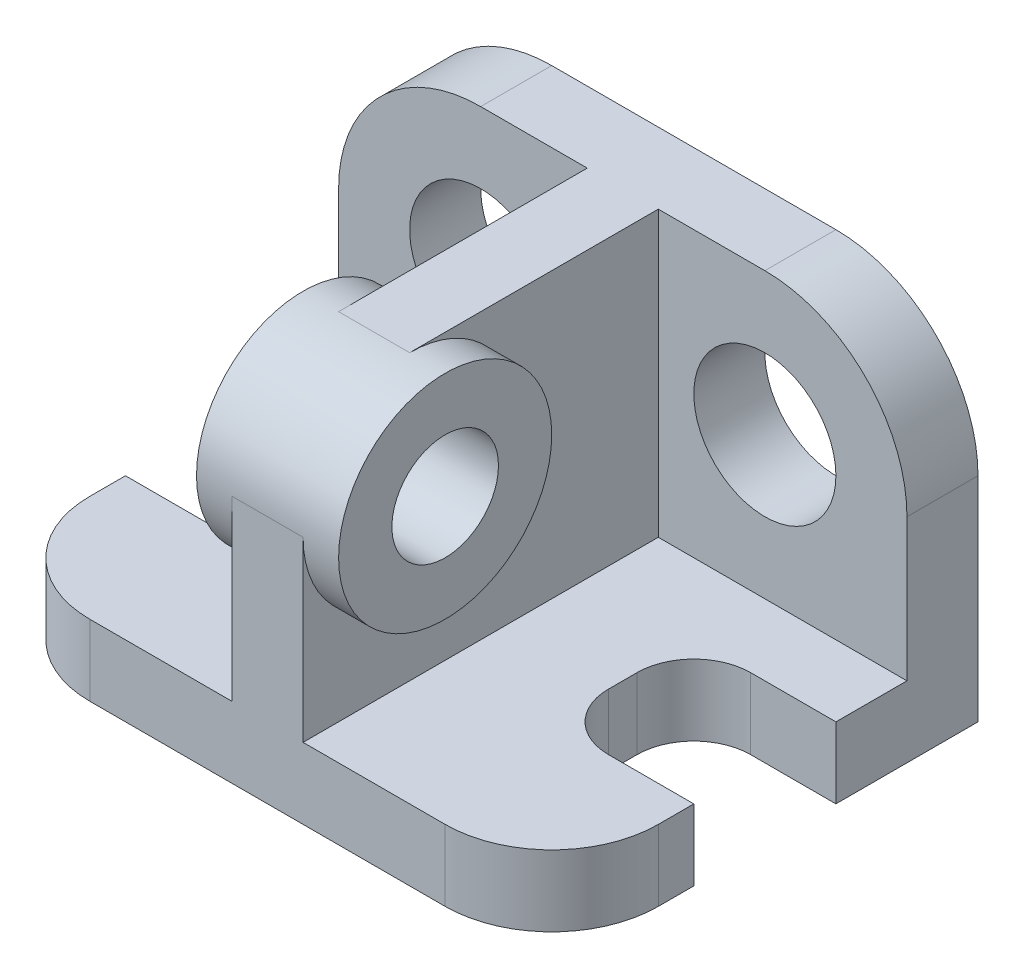
ISO-10303-21;
HEADER;
FILE_DESCRIPTION(('STEP AP214'),'2;1');
FILE_NAME('part.step','',(''),(''),'','','');
FILE_SCHEMA(('AUTOMOTIVE_DESIGN { 1 0 10303 214 1 1 1 1 }'));
ENDSEC;
DATA;
#1=APPLICATION_CONTEXT('core data for automotive mechanical design processes');
#2=APPLICATION_PROTOCOL_DEFINITION('international standard','automotive_design',2000,#1);
#3=PRODUCT_CONTEXT('',#1,'mechanical');
#4=PRODUCT('Part','Part','',(#3));
#5=PRODUCT_RELATED_PRODUCT_CATEGORY('part','',(#4));
#6=PRODUCT_DEFINITION_FORMATION('','',#4);
#7=PRODUCT_DEFINITION_CONTEXT('part definition',#1,'design');
#8=PRODUCT_DEFINITION('design','',#6,#7);
#9=PRODUCT_DEFINITION_SHAPE('','',#8);
#10=(LENGTH_UNIT() NAMED_UNIT(*) SI_UNIT(.MILLI.,.METRE.));
#11=(NAMED_UNIT(*) PLANE_ANGLE_UNIT() SI_UNIT($,.RADIAN.));
#12=(NAMED_UNIT(*) SI_UNIT($,.STERADIAN.) SOLID_ANGLE_UNIT());
#13=UNCERTAINTY_MEASURE_WITH_UNIT(LENGTH_MEASURE(1.E-05),#10,'distance_accuracy_value','');
#14=(GEOMETRIC_REPRESENTATION_CONTEXT(3) GLOBAL_UNCERTAINTY_ASSIGNED_CONTEXT((#13)) GLOBAL_UNIT_ASSIGNED_CONTEXT((#10,
#11,#12)) REPRESENTATION_CONTEXT('',''));
#15=CARTESIAN_POINT('',(0.,0.,0.));
#16=DIRECTION('',(0.,0.,1.));
#17=DIRECTION('',(1.,0.,0.));
#18=AXIS2_PLACEMENT_3D('',#15,#16,#17);
#19=CARTESIAN_POINT('',(-4.,-1.5,6.));
#20=DIRECTION('',(0.,-1.,0.));
#21=DIRECTION('',(0.,0.,-1.));
#22=AXIS2_PLACEMENT_3D('',#19,#20,#21);
#23=PLANE('',#22);
#24=DIRECTION('',(-1.,0.,0.));
#25=VECTOR('',#24,1.);
#26=CARTESIAN_POINT('',(-4.,-1.5,6.));
#27=LINE('',#26,#25);
#28=CARTESIAN_POINT('',(2.5,-1.5,6.));
#29=VERTEX_POINT('',#28);
#30=CARTESIAN_POINT('',(0.5,-1.5,6.));
#31=VERTEX_POINT('',#30);
#32=EDGE_CURVE('E285',#29,#31,#27,.T.);
#33=ORIENTED_EDGE('',*,*,#32,.F.);
#34=CARTESIAN_POINT('',(2.5,-1.5,4.5));
#35=DIRECTION('',(0.,-1.,0.));
#36=DIRECTION('',(0.,0.,-1.));
#37=AXIS2_PLACEMENT_3D('',#34,#35,#36);
#38=CIRCLE('',#37,1.5);
#39=CARTESIAN_POINT('',(4.,-1.5,4.5));
#40=VERTEX_POINT('',#39);
#41=EDGE_CURVE('E260',#29,#40,#38,.F.);
#42=ORIENTED_EDGE('',*,*,#41,.T.);
#43=DIRECTION('',(0.,0.,-1.));
#44=VECTOR('',#43,1.);
#45=CARTESIAN_POINT('',(4.,-1.5,6.));
#46=LINE('',#45,#44);
#47=CARTESIAN_POINT('',(4.,-1.5,4.));
#48=VERTEX_POINT('',#47);
#49=EDGE_CURVE('E283',#40,#48,#46,.T.);
#50=ORIENTED_EDGE('',*,*,#49,.T.);
#51=DIRECTION('',(1.,0.,0.));
#52=VECTOR('',#51,1.);
#53=CARTESIAN_POINT('',(4.,-1.5,4.));
#54=LINE('',#53,#52);
#55=CARTESIAN_POINT('',(2.8,-1.5,4.));
#56=VERTEX_POINT('',#55);
#57=EDGE_CURVE('E443',#56,#48,#54,.T.);
#58=ORIENTED_EDGE('',*,*,#57,.F.);
#59=CARTESIAN_POINT('',(2.8,-1.5,3.2));
#60=DIRECTION('',(0.,1.,0.));
#61=DIRECTION('',(0.,0.,-1.));
#62=AXIS2_PLACEMENT_3D('',#59,#60,#61);
#63=CIRCLE('',#62,0.8);
#64=CARTESIAN_POINT('',(2.,-1.5,3.2));
#65=VERTEX_POINT('',#64);
#66=EDGE_CURVE('E447',#65,#56,#63,.T.);
#67=ORIENTED_EDGE('',*,*,#66,.F.);
#68=DIRECTION('',(0.,0.,1.));
#69=VECTOR('',#68,1.);
#70=CARTESIAN_POINT('',(2.,-1.5,2.8));
#71=LINE('',#70,#69);
#72=CARTESIAN_POINT('',(2.,-1.5,2.8));
#73=VERTEX_POINT('',#72);
#74=EDGE_CURVE('E448',#73,#65,#71,.T.);
#75=ORIENTED_EDGE('',*,*,#74,.F.);
#76=CARTESIAN_POINT('',(2.8,-1.5,2.8));
#77=DIRECTION('',(0.,1.,0.));
#78=DIRECTION('',(0.,0.,-1.));
#79=AXIS2_PLACEMENT_3D('',#76,#77,#78);
#80=CIRCLE('',#79,0.8);
#81=CARTESIAN_POINT('',(2.8,-1.5,2.));
#82=VERTEX_POINT('',#81);
#83=EDGE_CURVE('E454',#82,#73,#80,.T.);
#84=ORIENTED_EDGE('',*,*,#83,.F.);
#85=DIRECTION('',(-1.,0.,0.));
#86=VECTOR('',#85,1.);
#87=CARTESIAN_POINT('',(4.,-1.5,2.));
#88=LINE('',#87,#86);
#89=CARTESIAN_POINT('',(4.,-1.5,2.));
#90=VERTEX_POINT('',#89);
#91=EDGE_CURVE('E406',#90,#82,#88,.T.);
#92=ORIENTED_EDGE('',*,*,#91,.F.);
#93=CARTESIAN_POINT('',(4.,-1.5,1.));
#94=VERTEX_POINT('',#93);
#95=EDGE_CURVE('E293',#90,#94,#46,.T.);
#96=ORIENTED_EDGE('',*,*,#95,.T.);
#97=DIRECTION('',(-1.,0.,0.));
#98=VECTOR('',#97,1.);
#99=CARTESIAN_POINT('',(-4.,-1.5,1.));
#100=LINE('',#99,#98);
#101=CARTESIAN_POINT('',(0.5,-1.5,1.));
#102=VERTEX_POINT('',#101);
#103=EDGE_CURVE('E273',#94,#102,#100,.T.);
#104=ORIENTED_EDGE('',*,*,#103,.T.);
#105=DIRECTION('',(0.,0.,-1.));
#106=VECTOR('',#105,1.);
#107=CARTESIAN_POINT('',(0.5,-1.5,1.));
#108=LINE('',#107,#106);
#109=EDGE_CURVE('E238',#31,#102,#108,.T.);
#110=ORIENTED_EDGE('',*,*,#109,.F.);
#111=EDGE_LOOP('',(#33,#42,#50,#58,#67,#75,#84,#92,#96,#104,#110));
#112=FACE_BOUND('',#111,.T.);
#113=ADVANCED_FACE('F39',(#112),#23,.F.);
#114=CARTESIAN_POINT('',(-2.,0.500000000000001,1.));
#115=DIRECTION('',(0.,0.,-1.));
#116=DIRECTION('',(-1.,0.,0.));
#117=AXIS2_PLACEMENT_3D('',#114,#115,#116);
#118=PLANE('',#117);
#119=CARTESIAN_POINT('',(2.,0.5,1.));
#120=DIRECTION('',(0.,0.,1.));
#121=DIRECTION('',(1.,0.,0.));
#122=AXIS2_PLACEMENT_3D('',#119,#120,#121);
#123=CIRCLE('',#122,1.);
#124=CARTESIAN_POINT('',(3.,0.5,1.));
#125=VERTEX_POINT('',#124);
#126=EDGE_CURVE('E295',#125,#125,#123,.T.);
#127=ORIENTED_EDGE('',*,*,#126,.F.);
#128=EDGE_LOOP('',(#127));
#129=FACE_BOUND('',#128,.T.);
#130=DIRECTION('',(0.,1.,0.));
#131=VECTOR('',#130,1.);
#132=CARTESIAN_POINT('',(0.5,2.5,1.));
#133=LINE('',#132,#131);
#134=CARTESIAN_POINT('',(0.5,2.5,1.));
#135=VERTEX_POINT('',#134);
#136=EDGE_CURVE('E383',#102,#135,#133,.T.);
#137=ORIENTED_EDGE('',*,*,#136,.F.);
#138=ORIENTED_EDGE('',*,*,#103,.F.);
#139=DIRECTION('',(0.,1.,0.));
#140=VECTOR('',#139,1.);
#141=CARTESIAN_POINT('',(4.,0.5,1.));
#142=LINE('',#141,#140);
#143=CARTESIAN_POINT('',(4.,0.5,1.));
#144=VERTEX_POINT('',#143);
#145=EDGE_CURVE('E307',#94,#144,#142,.T.);
#146=ORIENTED_EDGE('',*,*,#145,.T.);
#147=CARTESIAN_POINT('',(2.,0.5,1.));
#148=DIRECTION('',(0.,0.,1.));
#149=DIRECTION('',(1.,0.,0.));
#150=AXIS2_PLACEMENT_3D('',#147,#148,#149);
#151=CIRCLE('',#150,2.);
#152=CARTESIAN_POINT('',(2.,2.5,1.));
#153=VERTEX_POINT('',#152);
#154=EDGE_CURVE('E311',#144,#153,#151,.T.);
#155=ORIENTED_EDGE('',*,*,#154,.T.);
#156=DIRECTION('',(-1.,0.,0.));
#157=VECTOR('',#156,1.);
#158=CARTESIAN_POINT('',(-2.,2.5,1.));
#159=LINE('',#158,#157);
#160=EDGE_CURVE('E314',#153,#135,#159,.T.);
#161=ORIENTED_EDGE('',*,*,#160,.T.);
#162=EDGE_LOOP('',(#137,#138,#146,#155,#161));
#163=FACE_BOUND('',#162,.T.);
#164=ADVANCED_FACE('F481',(#129,#163),#118,.F.);
#165=CARTESIAN_POINT('',(4.,0.5,1.));
#166=DIRECTION('',(-1.,0.,0.));
#167=DIRECTION('',(0.,-1.,0.));
#168=AXIS2_PLACEMENT_3D('',#165,#166,#167);
#169=PLANE('',#168);
#170=DIRECTION('',(0.,1.,0.));
#171=VECTOR('',#170,1.);
#172=CARTESIAN_POINT('',(4.,-2.5,2.));
#173=LINE('',#172,#171);
#174=CARTESIAN_POINT('',(4.,-2.5,2.));
#175=VERTEX_POINT('',#174);
#176=EDGE_CURVE('E431',#175,#90,#173,.T.);
#177=ORIENTED_EDGE('',*,*,#176,.F.);
#178=DIRECTION('',(0.,0.,-1.));
#179=VECTOR('',#178,1.);
#180=CARTESIAN_POINT('',(4.,-2.5,1.));
#181=LINE('',#180,#179);
#182=CARTESIAN_POINT('',(4.,-2.5,0.));
#183=VERTEX_POINT('',#182);
#184=EDGE_CURVE('E325',#175,#183,#181,.T.);
#185=ORIENTED_EDGE('',*,*,#184,.T.);
#186=DIRECTION('',(0.,1.,0.));
#187=VECTOR('',#186,1.);
#188=CARTESIAN_POINT('',(4.,0.5,0.));
#189=LINE('',#188,#187);
#190=CARTESIAN_POINT('',(4.,0.5,0.));
#191=VERTEX_POINT('',#190);
#192=EDGE_CURVE('E306',#183,#191,#189,.T.);
#193=ORIENTED_EDGE('',*,*,#192,.T.);
#194=DIRECTION('',(0.,0.,-1.));
#195=VECTOR('',#194,1.);
#196=CARTESIAN_POINT('',(4.,0.5,1.));
#197=LINE('',#196,#195);
#198=EDGE_CURVE('E244',#144,#191,#197,.T.);
#199=ORIENTED_EDGE('',*,*,#198,.F.);
#200=ORIENTED_EDGE('',*,*,#145,.F.);
#201=ORIENTED_EDGE('',*,*,#95,.F.);
#202=EDGE_LOOP('',(#177,#185,#193,#199,#200,#201));
#203=FACE_BOUND('',#202,.T.);
#204=ADVANCED_FACE('F489',(#203),#169,.F.);
#205=CARTESIAN_POINT('',(-4.,0.500000000000001,1.));
#206=DIRECTION('',(1.,0.,0.));
#207=DIRECTION('',(0.,1.,0.));
#208=AXIS2_PLACEMENT_3D('',#205,#206,#207);
#209=PLANE('',#208);
#210=DIRECTION('',(0.,0.,-1.));
#211=VECTOR('',#210,1.);
#212=CARTESIAN_POINT('',(-4.,-2.5,1.));
#213=LINE('',#212,#211);
#214=CARTESIAN_POINT('',(-4.,-2.5,4.5));
#215=VERTEX_POINT('',#214);
#216=CARTESIAN_POINT('',(-4.,-2.5,4.));
#217=VERTEX_POINT('',#216);
#218=EDGE_CURVE('E336',#215,#217,#213,.T.);
#219=ORIENTED_EDGE('',*,*,#218,.F.);
#220=DIRECTION('',(0.,-1.,0.));
#221=VECTOR('',#220,1.);
#222=CARTESIAN_POINT('',(-4.,0.500000000000001,4.5));
#223=LINE('',#222,#221);
#224=CARTESIAN_POINT('',(-4.,-1.5,4.5));
#225=VERTEX_POINT('',#224);
#226=EDGE_CURVE('E50',#215,#225,#223,.F.);
#227=ORIENTED_EDGE('',*,*,#226,.T.);
#228=DIRECTION('',(0.,0.,-1.));
#229=VECTOR('',#228,1.);
#230=CARTESIAN_POINT('',(-4.,-1.5,6.));
#231=LINE('',#230,#229);
#232=CARTESIAN_POINT('',(-4.,-1.5,4.));
#233=VERTEX_POINT('',#232);
#234=EDGE_CURVE('E298',#225,#233,#231,.T.);
#235=ORIENTED_EDGE('',*,*,#234,.T.);
#236=DIRECTION('',(0.,1.,0.));
#237=VECTOR('',#236,1.);
#238=CARTESIAN_POINT('',(-4.,-2.5,4.));
#239=LINE('',#238,#237);
#240=EDGE_CURVE('E404',#217,#233,#239,.T.);
#241=ORIENTED_EDGE('',*,*,#240,.F.);
#242=EDGE_LOOP('',(#219,#227,#235,#241));
#243=FACE_BOUND('',#242,.T.);
#244=ADVANCED_FACE('F496',(#243),#209,.F.);
#245=ORIENTED_EDGE('',*,*,#234,.F.);
#246=CARTESIAN_POINT('',(-2.5,-1.5,4.5));
#247=DIRECTION('',(0.,-1.,0.));
#248=DIRECTION('',(0.,0.,-1.));
#249=AXIS2_PLACEMENT_3D('',#246,#247,#248);
#250=CIRCLE('',#249,1.5);
#251=CARTESIAN_POINT('',(-2.5,-1.5,6.));
#252=VERTEX_POINT('',#251);
#253=EDGE_CURVE('E11',#225,#252,#250,.F.);
#254=ORIENTED_EDGE('',*,*,#253,.T.);
#255=CARTESIAN_POINT('',(-0.5,-1.5,6.));
#256=VERTEX_POINT('',#255);
#257=EDGE_CURVE('E274',#256,#252,#27,.T.);
#258=ORIENTED_EDGE('',*,*,#257,.F.);
#259=DIRECTION('',(0.,0.,-1.));
#260=VECTOR('',#259,1.);
#261=CARTESIAN_POINT('',(-0.5,-1.5,1.));
#262=LINE('',#261,#260);
#263=CARTESIAN_POINT('',(-0.5,-1.5,1.));
#264=VERTEX_POINT('',#263);
#265=EDGE_CURVE('E222',#256,#264,#262,.T.);
#266=ORIENTED_EDGE('',*,*,#265,.T.);
#267=CARTESIAN_POINT('',(-4.,-1.5,1.));
#268=VERTEX_POINT('',#267);
#269=EDGE_CURVE('E380',#264,#268,#100,.T.);
#270=ORIENTED_EDGE('',*,*,#269,.T.);
#271=CARTESIAN_POINT('',(-4.,-1.5,2.));
#272=VERTEX_POINT('',#271);
#273=EDGE_CURVE('E373',#272,#268,#231,.T.);
#274=ORIENTED_EDGE('',*,*,#273,.F.);
#275=DIRECTION('',(-1.,0.,0.));
#276=VECTOR('',#275,1.);
#277=CARTESIAN_POINT('',(-4.,-1.5,2.));
#278=LINE('',#277,#276);
#279=CARTESIAN_POINT('',(-2.8,-1.5,2.));
#280=VERTEX_POINT('',#279);
#281=EDGE_CURVE('E394',#280,#272,#278,.T.);
#282=ORIENTED_EDGE('',*,*,#281,.F.);
#283=CARTESIAN_POINT('',(-2.8,-1.5,2.8));
#284=DIRECTION('',(0.,1.,0.));
#285=DIRECTION('',(0.,0.,1.));
#286=AXIS2_PLACEMENT_3D('',#283,#284,#285);
#287=CIRCLE('',#286,0.8);
#288=CARTESIAN_POINT('',(-2.,-1.5,2.8));
#289=VERTEX_POINT('',#288);
#290=EDGE_CURVE('E415',#289,#280,#287,.T.);
#291=ORIENTED_EDGE('',*,*,#290,.F.);
#292=DIRECTION('',(0.,0.,-1.));
#293=VECTOR('',#292,1.);
#294=CARTESIAN_POINT('',(-2.,-1.5,2.8));
#295=LINE('',#294,#293);
#296=CARTESIAN_POINT('',(-2.,-1.5,3.2));
#297=VERTEX_POINT('',#296);
#298=EDGE_CURVE('E413',#297,#289,#295,.T.);
#299=ORIENTED_EDGE('',*,*,#298,.F.);
#300=CARTESIAN_POINT('',(-2.8,-1.5,3.2));
#301=DIRECTION('',(0.,1.,0.));
#302=DIRECTION('',(0.,0.,1.));
#303=AXIS2_PLACEMENT_3D('',#300,#301,#302);
#304=CIRCLE('',#303,0.8);
#305=CARTESIAN_POINT('',(-2.8,-1.5,4.));
#306=VERTEX_POINT('',#305);
#307=EDGE_CURVE('E409',#306,#297,#304,.T.);
#308=ORIENTED_EDGE('',*,*,#307,.F.);
#309=DIRECTION('',(1.,0.,0.));
#310=VECTOR('',#309,1.);
#311=CARTESIAN_POINT('',(-4.,-1.5,4.));
#312=LINE('',#311,#310);
#313=EDGE_CURVE('E403',#233,#306,#312,.T.);
#314=ORIENTED_EDGE('',*,*,#313,.F.);
#315=EDGE_LOOP('',(#245,#254,#258,#266,#270,#274,#282,#291,#299,#308,#314));
#316=FACE_BOUND('',#315,.T.);
#317=ADVANCED_FACE('F474',(#316),#23,.F.);
#318=CARTESIAN_POINT('',(-2.,0.5,1.));
#319=DIRECTION('',(0.,0.,1.));
#320=DIRECTION('',(1.,0.,0.));
#321=AXIS2_PLACEMENT_3D('',#318,#319,#320);
#322=CIRCLE('',#321,1.);
#323=CARTESIAN_POINT('',(-1.,0.5,1.));
#324=VERTEX_POINT('',#323);
#325=EDGE_CURVE('E303',#324,#324,#322,.T.);
#326=ORIENTED_EDGE('',*,*,#325,.F.);
#327=EDGE_LOOP('',(#326));
#328=FACE_BOUND('',#327,.T.);
#329=ORIENTED_EDGE('',*,*,#269,.F.);
#330=DIRECTION('',(0.,1.,0.));
#331=VECTOR('',#330,1.);
#332=CARTESIAN_POINT('',(-0.5,2.5,1.));
#333=LINE('',#332,#331);
#334=CARTESIAN_POINT('',(-0.5,2.5,1.));
#335=VERTEX_POINT('',#334);
#336=EDGE_CURVE('E378',#264,#335,#333,.T.);
#337=ORIENTED_EDGE('',*,*,#336,.T.);
#338=CARTESIAN_POINT('',(-2.,2.5,1.));
#339=VERTEX_POINT('',#338);
#340=EDGE_CURVE('E313',#335,#339,#159,.T.);
#341=ORIENTED_EDGE('',*,*,#340,.T.);
#342=CARTESIAN_POINT('',(-2.,0.500000000000001,1.));
#343=DIRECTION('',(0.,0.,1.));
#344=DIRECTION('',(-1.,0.,0.));
#345=AXIS2_PLACEMENT_3D('',#342,#343,#344);
#346=CIRCLE('',#345,2.);
#347=CARTESIAN_POINT('',(-4.,0.500000000000001,1.));
#348=VERTEX_POINT('',#347);
#349=EDGE_CURVE('E320',#339,#348,#346,.T.);
#350=ORIENTED_EDGE('',*,*,#349,.T.);
#351=DIRECTION('',(0.,-1.,0.));
#352=VECTOR('',#351,1.);
#353=CARTESIAN_POINT('',(-4.,0.500000000000001,1.));
#354=LINE('',#353,#352);
#355=EDGE_CURVE('E316',#348,#268,#354,.T.);
#356=ORIENTED_EDGE('',*,*,#355,.T.);
#357=EDGE_LOOP('',(#329,#337,#341,#350,#356));
#358=FACE_BOUND('',#357,.T.);
#359=ADVANCED_FACE('F376',(#328,#358),#118,.F.);
#360=CARTESIAN_POINT('',(-2.,0.500000000000001,0.));
#361=DIRECTION('',(0.,0.,-1.));
#362=DIRECTION('',(-1.,0.,0.));
#363=AXIS2_PLACEMENT_3D('',#360,#361,#362);
#364=PLANE('',#363);
#365=CARTESIAN_POINT('',(-2.,0.5,0.));
#366=DIRECTION('',(0.,0.,1.));
#367=DIRECTION('',(1.,0.,0.));
#368=AXIS2_PLACEMENT_3D('',#365,#366,#367);
#369=CIRCLE('',#368,1.);
#370=CARTESIAN_POINT('',(-1.,0.5,0.));
#371=VERTEX_POINT('',#370);
#372=EDGE_CURVE('E301',#371,#371,#369,.T.);
#373=ORIENTED_EDGE('',*,*,#372,.T.);
#374=EDGE_LOOP('',(#373));
#375=FACE_BOUND('',#374,.T.);
#376=ORIENTED_EDGE('',*,*,#192,.F.);
#377=DIRECTION('',(1.,0.,0.));
#378=VECTOR('',#377,1.);
#379=CARTESIAN_POINT('',(-4.,-2.5,0.));
#380=LINE('',#379,#378);
#381=CARTESIAN_POINT('',(-4.,-2.5,0.));
#382=VERTEX_POINT('',#381);
#383=EDGE_CURVE('E315',#382,#183,#380,.T.);
#384=ORIENTED_EDGE('',*,*,#383,.F.);
#385=DIRECTION('',(0.,-1.,0.));
#386=VECTOR('',#385,1.);
#387=CARTESIAN_POINT('',(-4.,0.500000000000001,0.));
#388=LINE('',#387,#386);
#389=CARTESIAN_POINT('',(-4.,0.500000000000001,0.));
#390=VERTEX_POINT('',#389);
#391=EDGE_CURVE('E333',#390,#382,#388,.T.);
#392=ORIENTED_EDGE('',*,*,#391,.F.);
#393=CARTESIAN_POINT('',(-2.,0.500000000000001,0.));
#394=DIRECTION('',(0.,0.,1.));
#395=DIRECTION('',(-1.,0.,0.));
#396=AXIS2_PLACEMENT_3D('',#393,#394,#395);
#397=CIRCLE('',#396,2.);
#398=CARTESIAN_POINT('',(-2.,2.5,0.));
#399=VERTEX_POINT('',#398);
#400=EDGE_CURVE('E330',#399,#390,#397,.T.);
#401=ORIENTED_EDGE('',*,*,#400,.F.);
#402=DIRECTION('',(-1.,0.,0.));
#403=VECTOR('',#402,1.);
#404=CARTESIAN_POINT('',(-2.,2.5,0.));
#405=LINE('',#404,#403);
#406=CARTESIAN_POINT('',(2.,2.5,0.));
#407=VERTEX_POINT('',#406);
#408=EDGE_CURVE('E329',#407,#399,#405,.T.);
#409=ORIENTED_EDGE('',*,*,#408,.F.);
#410=CARTESIAN_POINT('',(2.,0.5,0.));
#411=DIRECTION('',(0.,0.,1.));
#412=DIRECTION('',(1.,0.,0.));
#413=AXIS2_PLACEMENT_3D('',#410,#411,#412);
#414=CIRCLE('',#413,2.);
#415=EDGE_CURVE('E323',#191,#407,#414,.T.);
#416=ORIENTED_EDGE('',*,*,#415,.F.);
#417=EDGE_LOOP('',(#376,#384,#392,#401,#409,#416));
#418=FACE_BOUND('',#417,.T.);
#419=CARTESIAN_POINT('',(2.,0.5,0.));
#420=DIRECTION('',(0.,0.,1.));
#421=DIRECTION('',(1.,0.,0.));
#422=AXIS2_PLACEMENT_3D('',#419,#420,#421);
#423=CIRCLE('',#422,1.);
#424=CARTESIAN_POINT('',(3.,0.5,0.));
#425=VERTEX_POINT('',#424);
#426=EDGE_CURVE('E289',#425,#425,#423,.T.);
#427=ORIENTED_EDGE('',*,*,#426,.T.);
#428=EDGE_LOOP('',(#427));
#429=FACE_BOUND('',#428,.T.);
#430=ADVANCED_FACE('F356',(#375,#418,#429),#364,.T.);
#431=ORIENTED_EDGE('',*,*,#49,.F.);
#432=DIRECTION('',(0.,1.,0.));
#433=VECTOR('',#432,1.);
#434=CARTESIAN_POINT('',(4.,0.5,4.5));
#435=LINE('',#434,#433);
#436=CARTESIAN_POINT('',(4.,-2.5,4.5));
#437=VERTEX_POINT('',#436);
#438=EDGE_CURVE('E256',#40,#437,#435,.F.);
#439=ORIENTED_EDGE('',*,*,#438,.T.);
#440=CARTESIAN_POINT('',(4.,-2.5,4.));
#441=VERTEX_POINT('',#440);
#442=EDGE_CURVE('E266',#437,#441,#181,.T.);
#443=ORIENTED_EDGE('',*,*,#442,.T.);
#444=DIRECTION('',(0.,1.,0.));
#445=VECTOR('',#444,1.);
#446=CARTESIAN_POINT('',(4.,-2.5,4.));
#447=LINE('',#446,#445);
#448=EDGE_CURVE('E287',#441,#48,#447,.T.);
#449=ORIENTED_EDGE('',*,*,#448,.T.);
#450=EDGE_LOOP('',(#431,#439,#443,#449));
#451=FACE_BOUND('',#450,.T.);
#452=ADVANCED_FACE('F290',(#451),#169,.F.);
#453=CARTESIAN_POINT('',(2.,0.5,1.));
#454=DIRECTION('',(0.,0.,-1.));
#455=DIRECTION('',(-1.,0.,0.));
#456=AXIS2_PLACEMENT_3D('',#453,#454,#455);
#457=CYLINDRICAL_SURFACE('',#456,2.);
#458=ORIENTED_EDGE('',*,*,#415,.T.);
#459=DIRECTION('',(0.,0.,-1.));
#460=VECTOR('',#459,1.);
#461=CARTESIAN_POINT('',(2.,2.5,1.));
#462=LINE('',#461,#460);
#463=EDGE_CURVE('E252',#153,#407,#462,.T.);
#464=ORIENTED_EDGE('',*,*,#463,.F.);
#465=ORIENTED_EDGE('',*,*,#154,.F.);
#466=ORIENTED_EDGE('',*,*,#198,.T.);
#467=EDGE_LOOP('',(#458,#464,#465,#466));
#468=FACE_BOUND('',#467,.T.);
#469=ADVANCED_FACE('F524',(#468),#457,.T.);
#470=CARTESIAN_POINT('',(-2.,2.5,1.));
#471=DIRECTION('',(0.,-1.,0.));
#472=DIRECTION('',(1.,0.,0.));
#473=AXIS2_PLACEMENT_3D('',#470,#471,#472);
#474=PLANE('',#473);
#475=ORIENTED_EDGE('',*,*,#408,.T.);
#476=DIRECTION('',(0.,0.,-1.));
#477=VECTOR('',#476,1.);
#478=CARTESIAN_POINT('',(-2.,2.5,1.));
#479=LINE('',#478,#477);
#480=EDGE_CURVE('E344',#339,#399,#479,.T.);
#481=ORIENTED_EDGE('',*,*,#480,.F.);
#482=ORIENTED_EDGE('',*,*,#340,.F.);
#483=DIRECTION('',(0.,0.,1.));
#484=VECTOR('',#483,1.);
#485=CARTESIAN_POINT('',(-0.5,2.5,1.));
#486=LINE('',#485,#484);
#487=CARTESIAN_POINT('',(-0.5,2.5,4.5));
#488=VERTEX_POINT('',#487);
#489=EDGE_CURVE('E227',#335,#488,#486,.T.);
#490=ORIENTED_EDGE('',*,*,#489,.T.);
#491=DIRECTION('',(-1.,0.,0.));
#492=VECTOR('',#491,1.);
#493=CARTESIAN_POINT('',(0.5,2.5,4.5));
#494=LINE('',#493,#492);
#495=CARTESIAN_POINT('',(0.5,2.5,4.5));
#496=VERTEX_POINT('',#495);
#497=EDGE_CURVE('E240',#496,#488,#494,.T.);
#498=ORIENTED_EDGE('',*,*,#497,.F.);
#499=DIRECTION('',(0.,0.,1.));
#500=VECTOR('',#499,1.);
#501=CARTESIAN_POINT('',(0.5,2.5,1.));
#502=LINE('',#501,#500);
#503=EDGE_CURVE('E547',#135,#496,#502,.T.);
#504=ORIENTED_EDGE('',*,*,#503,.F.);
#505=ORIENTED_EDGE('',*,*,#160,.F.);
#506=ORIENTED_EDGE('',*,*,#463,.T.);
#507=EDGE_LOOP('',(#475,#481,#482,#490,#498,#504,#505,#506));
#508=FACE_BOUND('',#507,.T.);
#509=ADVANCED_FACE('F346',(#508),#474,.F.);
#510=CARTESIAN_POINT('',(-2.,0.500000000000001,1.));
#511=DIRECTION('',(0.,0.,-1.));
#512=DIRECTION('',(-1.,0.,0.));
#513=AXIS2_PLACEMENT_3D('',#510,#511,#512);
#514=CYLINDRICAL_SURFACE('',#513,2.);
#515=ORIENTED_EDGE('',*,*,#400,.T.);
#516=DIRECTION('',(0.,0.,-1.));
#517=VECTOR('',#516,1.);
#518=CARTESIAN_POINT('',(-4.,0.500000000000001,1.));
#519=LINE('',#518,#517);
#520=EDGE_CURVE('E338',#348,#390,#519,.T.);
#521=ORIENTED_EDGE('',*,*,#520,.F.);
#522=ORIENTED_EDGE('',*,*,#349,.F.);
#523=ORIENTED_EDGE('',*,*,#480,.T.);
#524=EDGE_LOOP('',(#515,#521,#522,#523));
#525=FACE_BOUND('',#524,.T.);
#526=ADVANCED_FACE('F364',(#525),#514,.T.);
#527=CARTESIAN_POINT('',(-4.,-2.5,2.));
#528=VERTEX_POINT('',#527);
#529=EDGE_CURVE('E340',#528,#382,#213,.T.);
#530=ORIENTED_EDGE('',*,*,#529,.F.);
#531=DIRECTION('',(0.,1.,0.));
#532=VECTOR('',#531,1.);
#533=CARTESIAN_POINT('',(-4.,-2.5,2.));
#534=LINE('',#533,#532);
#535=EDGE_CURVE('E416',#528,#272,#534,.T.);
#536=ORIENTED_EDGE('',*,*,#535,.T.);
#537=ORIENTED_EDGE('',*,*,#273,.T.);
#538=ORIENTED_EDGE('',*,*,#355,.F.);
#539=ORIENTED_EDGE('',*,*,#520,.T.);
#540=ORIENTED_EDGE('',*,*,#391,.T.);
#541=EDGE_LOOP('',(#530,#536,#537,#538,#539,#540));
#542=FACE_BOUND('',#541,.T.);
#543=ADVANCED_FACE('F367',(#542),#209,.F.);
#544=CARTESIAN_POINT('',(-4.,-2.5,1.));
#545=DIRECTION('',(0.,1.,0.));
#546=DIRECTION('',(0.,0.,1.));
#547=AXIS2_PLACEMENT_3D('',#544,#545,#546);
#548=PLANE('',#547);
#549=ORIENTED_EDGE('',*,*,#442,.F.);
#550=CARTESIAN_POINT('',(2.5,-2.5,4.5));
#551=DIRECTION('',(0.,1.,0.));
#552=DIRECTION('',(0.,0.,1.));
#553=AXIS2_PLACEMENT_3D('',#550,#551,#552);
#554=CIRCLE('',#553,1.5);
#555=CARTESIAN_POINT('',(2.5,-2.5,6.));
#556=VERTEX_POINT('',#555);
#557=EDGE_CURVE('E264',#437,#556,#554,.F.);
#558=ORIENTED_EDGE('',*,*,#557,.T.);
#559=DIRECTION('',(1.,0.,0.));
#560=VECTOR('',#559,1.);
#561=CARTESIAN_POINT('',(-4.,-2.5,6.));
#562=LINE('',#561,#560);
#563=CARTESIAN_POINT('',(-2.5,-2.5,6.));
#564=VERTEX_POINT('',#563);
#565=EDGE_CURVE('E268',#564,#556,#562,.T.);
#566=ORIENTED_EDGE('',*,*,#565,.F.);
#567=CARTESIAN_POINT('',(-2.5,-2.5,4.5));
#568=DIRECTION('',(0.,1.,0.));
#569=DIRECTION('',(0.,0.,1.));
#570=AXIS2_PLACEMENT_3D('',#567,#568,#569);
#571=CIRCLE('',#570,1.5);
#572=EDGE_CURVE('E62',#564,#215,#571,.F.);
#573=ORIENTED_EDGE('',*,*,#572,.T.);
#574=ORIENTED_EDGE('',*,*,#218,.T.);
#575=DIRECTION('',(1.,0.,0.));
#576=VECTOR('',#575,1.);
#577=CARTESIAN_POINT('',(-4.,-2.5,4.));
#578=LINE('',#577,#576);
#579=CARTESIAN_POINT('',(-2.8,-2.5,4.));
#580=VERTEX_POINT('',#579);
#581=EDGE_CURVE('E389',#217,#580,#578,.T.);
#582=ORIENTED_EDGE('',*,*,#581,.T.);
#583=CARTESIAN_POINT('',(-2.8,-2.5,3.2));
#584=DIRECTION('',(0.,1.,0.));
#585=DIRECTION('',(0.,0.,1.));
#586=AXIS2_PLACEMENT_3D('',#583,#584,#585);
#587=CIRCLE('',#586,0.8);
#588=CARTESIAN_POINT('',(-2.,-2.5,3.2));
#589=VERTEX_POINT('',#588);
#590=EDGE_CURVE('E393',#580,#589,#587,.T.);
#591=ORIENTED_EDGE('',*,*,#590,.T.);
#592=DIRECTION('',(0.,0.,-1.));
#593=VECTOR('',#592,1.);
#594=CARTESIAN_POINT('',(-2.,-2.5,2.8));
#595=LINE('',#594,#593);
#596=CARTESIAN_POINT('',(-2.,-2.5,2.8));
#597=VERTEX_POINT('',#596);
#598=EDGE_CURVE('E391',#589,#597,#595,.T.);
#599=ORIENTED_EDGE('',*,*,#598,.T.);
#600=CARTESIAN_POINT('',(-2.8,-2.5,2.8));
#601=DIRECTION('',(0.,1.,0.));
#602=DIRECTION('',(0.,0.,1.));
#603=AXIS2_PLACEMENT_3D('',#600,#601,#602);
#604=CIRCLE('',#603,0.8);
#605=CARTESIAN_POINT('',(-2.8,-2.5,2.));
#606=VERTEX_POINT('',#605);
#607=EDGE_CURVE('E396',#597,#606,#604,.T.);
#608=ORIENTED_EDGE('',*,*,#607,.T.);
#609=DIRECTION('',(-1.,0.,0.));
#610=VECTOR('',#609,1.);
#611=CARTESIAN_POINT('',(-4.,-2.5,2.));
#612=LINE('',#611,#610);
#613=EDGE_CURVE('E402',#606,#528,#612,.T.);
#614=ORIENTED_EDGE('',*,*,#613,.T.);
#615=ORIENTED_EDGE('',*,*,#529,.T.);
#616=ORIENTED_EDGE('',*,*,#383,.T.);
#617=ORIENTED_EDGE('',*,*,#184,.F.);
#618=DIRECTION('',(-1.,0.,0.));
#619=VECTOR('',#618,1.);
#620=CARTESIAN_POINT('',(4.,-2.5,2.));
#621=LINE('',#620,#619);
#622=CARTESIAN_POINT('',(2.8,-2.5,2.));
#623=VERTEX_POINT('',#622);
#624=EDGE_CURVE('E450',#175,#623,#621,.T.);
#625=ORIENTED_EDGE('',*,*,#624,.T.);
#626=CARTESIAN_POINT('',(2.8,-2.5,2.8));
#627=DIRECTION('',(0.,1.,0.));
#628=DIRECTION('',(0.,0.,-1.));
#629=AXIS2_PLACEMENT_3D('',#626,#627,#628);
#630=CIRCLE('',#629,0.8);
#631=CARTESIAN_POINT('',(2.,-2.5,2.8));
#632=VERTEX_POINT('',#631);
#633=EDGE_CURVE('E462',#623,#632,#630,.T.);
#634=ORIENTED_EDGE('',*,*,#633,.T.);
#635=DIRECTION('',(0.,0.,1.));
#636=VECTOR('',#635,1.);
#637=CARTESIAN_POINT('',(2.,-2.5,2.8));
#638=LINE('',#637,#636);
#639=CARTESIAN_POINT('',(2.,-2.5,3.2));
#640=VERTEX_POINT('',#639);
#641=EDGE_CURVE('E463',#632,#640,#638,.T.);
#642=ORIENTED_EDGE('',*,*,#641,.T.);
#643=CARTESIAN_POINT('',(2.8,-2.5,3.2));
#644=DIRECTION('',(0.,1.,0.));
#645=DIRECTION('',(0.,0.,-1.));
#646=AXIS2_PLACEMENT_3D('',#643,#644,#645);
#647=CIRCLE('',#646,0.8);
#648=CARTESIAN_POINT('',(2.8,-2.5,4.));
#649=VERTEX_POINT('',#648);
#650=EDGE_CURVE('E457',#640,#649,#647,.T.);
#651=ORIENTED_EDGE('',*,*,#650,.T.);
#652=DIRECTION('',(1.,0.,0.));
#653=VECTOR('',#652,1.);
#654=CARTESIAN_POINT('',(4.,-2.5,4.));
#655=LINE('',#654,#653);
#656=EDGE_CURVE('E433',#649,#441,#655,.T.);
#657=ORIENTED_EDGE('',*,*,#656,.T.);
#658=EDGE_LOOP('',(#549,#558,#566,#573,#574,#582,#591,#599,#608,#614,#615,#616,#617,#625,#634,
#642,#651,#657));
#659=FACE_BOUND('',#658,.T.);
#660=ADVANCED_FACE('F261',(#659),#548,.F.);
#661=CARTESIAN_POINT('',(-2.,0.5,1.));
#662=DIRECTION('',(0.,0.,-1.));
#663=DIRECTION('',(-1.,0.,0.));
#664=AXIS2_PLACEMENT_3D('',#661,#662,#663);
#665=CYLINDRICAL_SURFACE('',#664,1.);
#666=ORIENTED_EDGE('',*,*,#325,.T.);
#667=EDGE_LOOP('',(#666));
#668=FACE_BOUND('',#667,.T.);
#669=ORIENTED_EDGE('',*,*,#372,.F.);
#670=EDGE_LOOP('',(#669));
#671=FACE_BOUND('',#670,.T.);
#672=ADVANCED_FACE('F513',(#668,#671),#665,.F.);
#673=CARTESIAN_POINT('',(2.,0.5,1.));
#674=DIRECTION('',(0.,0.,-1.));
#675=DIRECTION('',(-1.,0.,0.));
#676=AXIS2_PLACEMENT_3D('',#673,#674,#675);
#677=CYLINDRICAL_SURFACE('',#676,1.);
#678=ORIENTED_EDGE('',*,*,#126,.T.);
#679=EDGE_LOOP('',(#678));
#680=FACE_BOUND('',#679,.T.);
#681=ORIENTED_EDGE('',*,*,#426,.F.);
#682=EDGE_LOOP('',(#681));
#683=FACE_BOUND('',#682,.T.);
#684=ADVANCED_FACE('F531',(#680,#683),#677,.F.);
#685=CARTESIAN_POINT('',(0.,0.,6.));
#686=DIRECTION('',(0.,0.,-1.));
#687=DIRECTION('',(-1.,0.,0.));
#688=AXIS2_PLACEMENT_3D('',#685,#686,#687);
#689=PLANE('',#688);
#690=ORIENTED_EDGE('',*,*,#565,.T.);
#691=DIRECTION('',(0.,1.,0.));
#692=VECTOR('',#691,1.);
#693=CARTESIAN_POINT('',(2.5,0.,6.));
#694=LINE('',#693,#692);
#695=EDGE_CURVE('E247',#556,#29,#694,.T.);
#696=ORIENTED_EDGE('',*,*,#695,.T.);
#697=ORIENTED_EDGE('',*,*,#32,.T.);
#698=DIRECTION('',(0.,-1.,0.));
#699=VECTOR('',#698,1.);
#700=CARTESIAN_POINT('',(0.5,1.,6.));
#701=LINE('',#700,#699);
#702=CARTESIAN_POINT('',(0.5,1.,6.));
#703=VERTEX_POINT('',#702);
#704=EDGE_CURVE('E232',#703,#31,#701,.T.);
#705=ORIENTED_EDGE('',*,*,#704,.F.);
#706=DIRECTION('',(-1.,0.,0.));
#707=VECTOR('',#706,1.);
#708=CARTESIAN_POINT('',(0.5,1.,6.));
#709=LINE('',#708,#707);
#710=CARTESIAN_POINT('',(-0.5,1.,6.));
#711=VERTEX_POINT('',#710);
#712=EDGE_CURVE('E233',#703,#711,#709,.T.);
#713=ORIENTED_EDGE('',*,*,#712,.T.);
#714=DIRECTION('',(0.,-1.,0.));
#715=VECTOR('',#714,1.);
#716=CARTESIAN_POINT('',(-0.5,1.,6.));
#717=LINE('',#716,#715);
#718=EDGE_CURVE('E218',#711,#256,#717,.T.);
#719=ORIENTED_EDGE('',*,*,#718,.T.);
#720=ORIENTED_EDGE('',*,*,#257,.T.);
#721=DIRECTION('',(0.,-1.,0.));
#722=VECTOR('',#721,1.);
#723=CARTESIAN_POINT('',(-2.5,0.,6.));
#724=LINE('',#723,#722);
#725=EDGE_CURVE('E242',#252,#564,#724,.T.);
#726=ORIENTED_EDGE('',*,*,#725,.T.);
#727=EDGE_LOOP('',(#690,#696,#697,#705,#713,#719,#720,#726));
#728=FACE_BOUND('',#727,.T.);
#729=ADVANCED_FACE('F231',(#728),#689,.F.);
#730=CARTESIAN_POINT('',(4.,-2.5,4.));
#731=DIRECTION('',(0.,0.,1.));
#732=DIRECTION('',(1.,0.,0.));
#733=AXIS2_PLACEMENT_3D('',#730,#731,#732);
#734=PLANE('',#733);
#735=ORIENTED_EDGE('',*,*,#57,.T.);
#736=ORIENTED_EDGE('',*,*,#448,.F.);
#737=ORIENTED_EDGE('',*,*,#656,.F.);
#738=DIRECTION('',(0.,1.,0.));
#739=VECTOR('',#738,1.);
#740=CARTESIAN_POINT('',(2.8,-2.5,4.));
#741=LINE('',#740,#739);
#742=EDGE_CURVE('E441',#649,#56,#741,.T.);
#743=ORIENTED_EDGE('',*,*,#742,.T.);
#744=EDGE_LOOP('',(#735,#736,#737,#743));
#745=FACE_BOUND('',#744,.T.);
#746=ADVANCED_FACE('F538',(#745),#734,.F.);
#747=CARTESIAN_POINT('',(2.8,-2.5,3.2));
#748=DIRECTION('',(0.,1.,0.));
#749=DIRECTION('',(0.,0.,1.));
#750=AXIS2_PLACEMENT_3D('',#747,#748,#749);
#751=CYLINDRICAL_SURFACE('',#750,0.8);
#752=ORIENTED_EDGE('',*,*,#66,.T.);
#753=ORIENTED_EDGE('',*,*,#742,.F.);
#754=ORIENTED_EDGE('',*,*,#650,.F.);
#755=DIRECTION('',(0.,1.,0.));
#756=VECTOR('',#755,1.);
#757=CARTESIAN_POINT('',(2.,-2.5,3.2));
#758=LINE('',#757,#756);
#759=EDGE_CURVE('E437',#640,#65,#758,.T.);
#760=ORIENTED_EDGE('',*,*,#759,.T.);
#761=EDGE_LOOP('',(#752,#753,#754,#760));
#762=FACE_BOUND('',#761,.T.);
#763=ADVANCED_FACE('F623',(#762),#751,.F.);
#764=CARTESIAN_POINT('',(2.,-2.5,2.8));
#765=DIRECTION('',(-1.,0.,0.));
#766=DIRECTION('',(0.,0.,1.));
#767=AXIS2_PLACEMENT_3D('',#764,#765,#766);
#768=PLANE('',#767);
#769=ORIENTED_EDGE('',*,*,#74,.T.);
#770=ORIENTED_EDGE('',*,*,#759,.F.);
#771=ORIENTED_EDGE('',*,*,#641,.F.);
#772=DIRECTION('',(0.,1.,0.));
#773=VECTOR('',#772,1.);
#774=CARTESIAN_POINT('',(2.,-2.5,2.8));
#775=LINE('',#774,#773);
#776=EDGE_CURVE('E436',#632,#73,#775,.T.);
#777=ORIENTED_EDGE('',*,*,#776,.T.);
#778=EDGE_LOOP('',(#769,#770,#771,#777));
#779=FACE_BOUND('',#778,.T.);
#780=ADVANCED_FACE('F617',(#779),#768,.F.);
#781=CARTESIAN_POINT('',(2.8,-2.5,2.8));
#782=DIRECTION('',(0.,1.,0.));
#783=DIRECTION('',(0.,0.,1.));
#784=AXIS2_PLACEMENT_3D('',#781,#782,#783);
#785=CYLINDRICAL_SURFACE('',#784,0.8);
#786=ORIENTED_EDGE('',*,*,#83,.T.);
#787=ORIENTED_EDGE('',*,*,#776,.F.);
#788=ORIENTED_EDGE('',*,*,#633,.F.);
#789=DIRECTION('',(0.,1.,0.));
#790=VECTOR('',#789,1.);
#791=CARTESIAN_POINT('',(2.8,-2.5,2.));
#792=LINE('',#791,#790);
#793=EDGE_CURVE('E432',#623,#82,#792,.T.);
#794=ORIENTED_EDGE('',*,*,#793,.T.);
#795=EDGE_LOOP('',(#786,#787,#788,#794));
#796=FACE_BOUND('',#795,.T.);
#797=ADVANCED_FACE('F611',(#796),#785,.F.);
#798=CARTESIAN_POINT('',(4.,-2.5,2.));
#799=DIRECTION('',(0.,0.,-1.));
#800=DIRECTION('',(-1.,0.,0.));
#801=AXIS2_PLACEMENT_3D('',#798,#799,#800);
#802=PLANE('',#801);
#803=ORIENTED_EDGE('',*,*,#91,.T.);
#804=ORIENTED_EDGE('',*,*,#793,.F.);
#805=ORIENTED_EDGE('',*,*,#624,.F.);
#806=ORIENTED_EDGE('',*,*,#176,.T.);
#807=EDGE_LOOP('',(#803,#804,#805,#806));
#808=FACE_BOUND('',#807,.T.);
#809=ADVANCED_FACE('F594',(#808),#802,.F.);
#810=CARTESIAN_POINT('',(-4.,-2.5,2.));
#811=DIRECTION('',(0.,0.,-1.));
#812=DIRECTION('',(-1.,0.,0.));
#813=AXIS2_PLACEMENT_3D('',#810,#811,#812);
#814=PLANE('',#813);
#815=ORIENTED_EDGE('',*,*,#281,.T.);
#816=ORIENTED_EDGE('',*,*,#535,.F.);
#817=ORIENTED_EDGE('',*,*,#613,.F.);
#818=DIRECTION('',(0.,1.,0.));
#819=VECTOR('',#818,1.);
#820=CARTESIAN_POINT('',(-2.8,-2.5,2.));
#821=LINE('',#820,#819);
#822=EDGE_CURVE('E419',#606,#280,#821,.T.);
#823=ORIENTED_EDGE('',*,*,#822,.T.);
#824=EDGE_LOOP('',(#815,#816,#817,#823));
#825=FACE_BOUND('',#824,.T.);
#826=ADVANCED_FACE('F593',(#825),#814,.F.);
#827=CARTESIAN_POINT('',(-2.8,-2.5,2.8));
#828=DIRECTION('',(0.,1.,0.));
#829=DIRECTION('',(0.,0.,1.));
#830=AXIS2_PLACEMENT_3D('',#827,#828,#829);
#831=CYLINDRICAL_SURFACE('',#830,0.8);
#832=ORIENTED_EDGE('',*,*,#290,.T.);
#833=ORIENTED_EDGE('',*,*,#822,.F.);
#834=ORIENTED_EDGE('',*,*,#607,.F.);
#835=DIRECTION('',(0.,1.,0.));
#836=VECTOR('',#835,1.);
#837=CARTESIAN_POINT('',(-2.,-2.5,2.8));
#838=LINE('',#837,#836);
#839=EDGE_CURVE('E422',#597,#289,#838,.T.);
#840=ORIENTED_EDGE('',*,*,#839,.T.);
#841=EDGE_LOOP('',(#832,#833,#834,#840));
#842=FACE_BOUND('',#841,.T.);
#843=ADVANCED_FACE('F592',(#842),#831,.F.);
#844=CARTESIAN_POINT('',(-2.,-2.5,2.8));
#845=DIRECTION('',(1.,0.,0.));
#846=DIRECTION('',(0.,0.,-1.));
#847=AXIS2_PLACEMENT_3D('',#844,#845,#846);
#848=PLANE('',#847);
#849=ORIENTED_EDGE('',*,*,#298,.T.);
#850=ORIENTED_EDGE('',*,*,#839,.F.);
#851=ORIENTED_EDGE('',*,*,#598,.F.);
#852=DIRECTION('',(0.,1.,0.));
#853=VECTOR('',#852,1.);
#854=CARTESIAN_POINT('',(-2.,-2.5,3.2));
#855=LINE('',#854,#853);
#856=EDGE_CURVE('E425',#589,#297,#855,.T.);
#857=ORIENTED_EDGE('',*,*,#856,.T.);
#858=EDGE_LOOP('',(#849,#850,#851,#857));
#859=FACE_BOUND('',#858,.T.);
#860=ADVANCED_FACE('F599',(#859),#848,.F.);
#861=CARTESIAN_POINT('',(-2.8,-2.5,3.2));
#862=DIRECTION('',(0.,1.,0.));
#863=DIRECTION('',(0.,0.,1.));
#864=AXIS2_PLACEMENT_3D('',#861,#862,#863);
#865=CYLINDRICAL_SURFACE('',#864,0.8);
#866=ORIENTED_EDGE('',*,*,#307,.T.);
#867=ORIENTED_EDGE('',*,*,#856,.F.);
#868=ORIENTED_EDGE('',*,*,#590,.F.);
#869=DIRECTION('',(0.,1.,0.));
#870=VECTOR('',#869,1.);
#871=CARTESIAN_POINT('',(-2.8,-2.5,4.));
#872=LINE('',#871,#870);
#873=EDGE_CURVE('E430',#580,#306,#872,.T.);
#874=ORIENTED_EDGE('',*,*,#873,.T.);
#875=EDGE_LOOP('',(#866,#867,#868,#874));
#876=FACE_BOUND('',#875,.T.);
#877=ADVANCED_FACE('F604',(#876),#865,.F.);
#878=CARTESIAN_POINT('',(-4.,-2.5,4.));
#879=DIRECTION('',(0.,0.,1.));
#880=DIRECTION('',(1.,0.,0.));
#881=AXIS2_PLACEMENT_3D('',#878,#879,#880);
#882=PLANE('',#881);
#883=ORIENTED_EDGE('',*,*,#313,.T.);
#884=ORIENTED_EDGE('',*,*,#873,.F.);
#885=ORIENTED_EDGE('',*,*,#581,.F.);
#886=ORIENTED_EDGE('',*,*,#240,.T.);
#887=EDGE_LOOP('',(#883,#884,#885,#886));
#888=FACE_BOUND('',#887,.T.);
#889=ADVANCED_FACE('F586',(#888),#882,.F.);
#890=CARTESIAN_POINT('',(0.5,1.,4.5));
#891=DIRECTION('',(-1.,0.,0.));
#892=DIRECTION('',(0.,0.,1.));
#893=AXIS2_PLACEMENT_3D('',#890,#891,#892);
#894=CYLINDRICAL_SURFACE('',#893,1.5);
#895=ORIENTED_EDGE('',*,*,#497,.T.);
#896=CARTESIAN_POINT('',(-0.5,1.,4.5));
#897=DIRECTION('',(1.,0.,0.));
#898=DIRECTION('',(0.,0.,-1.));
#899=AXIS2_PLACEMENT_3D('',#896,#897,#898);
#900=CIRCLE('',#899,1.5);
#901=EDGE_CURVE('E223',#488,#711,#900,.F.);
#902=ORIENTED_EDGE('',*,*,#901,.T.);
#903=ORIENTED_EDGE('',*,*,#712,.F.);
#904=CARTESIAN_POINT('',(0.5,1.,4.5));
#905=DIRECTION('',(1.,0.,0.));
#906=DIRECTION('',(0.,0.,-1.));
#907=AXIS2_PLACEMENT_3D('',#904,#905,#906);
#908=CIRCLE('',#907,1.5);
#909=EDGE_CURVE('E382',#496,#703,#908,.F.);
#910=ORIENTED_EDGE('',*,*,#909,.F.);
#911=EDGE_LOOP('',(#895,#902,#903,#910));
#912=FACE_BOUND('',#911,.T.);
#913=CARTESIAN_POINT('',(-1.,1.,4.5));
#914=DIRECTION('',(1.,0.,0.));
#915=DIRECTION('',(0.,0.,-1.));
#916=AXIS2_PLACEMENT_3D('',#913,#914,#915);
#917=CIRCLE('',#916,1.5);
#918=CARTESIAN_POINT('',(-1.,1.,3.));
#919=VERTEX_POINT('',#918);
#920=EDGE_CURVE('E556',#919,#919,#917,.T.);
#921=ORIENTED_EDGE('',*,*,#920,.T.);
#922=EDGE_LOOP('',(#921));
#923=FACE_BOUND('',#922,.T.);
#924=CARTESIAN_POINT('',(1.,1.,4.5));
#925=DIRECTION('',(1.,0.,0.));
#926=DIRECTION('',(0.,0.,-1.));
#927=AXIS2_PLACEMENT_3D('',#924,#925,#926);
#928=CIRCLE('',#927,1.5);
#929=CARTESIAN_POINT('',(1.,1.,3.));
#930=VERTEX_POINT('',#929);
#931=EDGE_CURVE('E558',#930,#930,#928,.T.);
#932=ORIENTED_EDGE('',*,*,#931,.F.);
#933=EDGE_LOOP('',(#932));
#934=FACE_BOUND('',#933,.T.);
#935=ADVANCED_FACE('F241',(#912,#923,#934),#894,.T.);
#936=CARTESIAN_POINT('',(0.5,1.,4.5));
#937=DIRECTION('',(1.,0.,0.));
#938=DIRECTION('',(0.,0.,-1.));
#939=AXIS2_PLACEMENT_3D('',#936,#937,#938);
#940=PLANE('',#939);
#941=ORIENTED_EDGE('',*,*,#503,.T.);
#942=ORIENTED_EDGE('',*,*,#909,.T.);
#943=ORIENTED_EDGE('',*,*,#704,.T.);
#944=ORIENTED_EDGE('',*,*,#109,.T.);
#945=ORIENTED_EDGE('',*,*,#136,.T.);
#946=EDGE_LOOP('',(#941,#942,#943,#944,#945));
#947=FACE_BOUND('',#946,.T.);
#948=ADVANCED_FACE('F554',(#947),#940,.T.);
#949=CARTESIAN_POINT('',(-0.5,1.,4.5));
#950=DIRECTION('',(1.,0.,0.));
#951=DIRECTION('',(0.,0.,-1.));
#952=AXIS2_PLACEMENT_3D('',#949,#950,#951);
#953=PLANE('',#952);
#954=ORIENTED_EDGE('',*,*,#901,.F.);
#955=ORIENTED_EDGE('',*,*,#489,.F.);
#956=ORIENTED_EDGE('',*,*,#336,.F.);
#957=ORIENTED_EDGE('',*,*,#265,.F.);
#958=ORIENTED_EDGE('',*,*,#718,.F.);
#959=EDGE_LOOP('',(#954,#955,#956,#957,#958));
#960=FACE_BOUND('',#959,.T.);
#961=ADVANCED_FACE('F217',(#960),#953,.F.);
#962=CARTESIAN_POINT('',(-1.,1.,4.5));
#963=DIRECTION('',(1.,0.,0.));
#964=DIRECTION('',(0.,0.,-1.));
#965=AXIS2_PLACEMENT_3D('',#962,#963,#964);
#966=PLANE('',#965);
#967=ORIENTED_EDGE('',*,*,#920,.F.);
#968=EDGE_LOOP('',(#967));
#969=FACE_BOUND('',#968,.T.);
#970=CARTESIAN_POINT('',(-1.,1.,4.5));
#971=DIRECTION('',(1.,0.,0.));
#972=DIRECTION('',(0.,0.,-1.));
#973=AXIS2_PLACEMENT_3D('',#970,#971,#972);
#974=CIRCLE('',#973,0.75);
#975=CARTESIAN_POINT('',(-1.,1.,3.75));
#976=VERTEX_POINT('',#975);
#977=EDGE_CURVE('E564',#976,#976,#974,.T.);
#978=ORIENTED_EDGE('',*,*,#977,.T.);
#979=EDGE_LOOP('',(#978));
#980=FACE_BOUND('',#979,.T.);
#981=ADVANCED_FACE('F579',(#969,#980),#966,.F.);
#982=CARTESIAN_POINT('',(1.,1.,4.5));
#983=DIRECTION('',(-1.,0.,0.));
#984=DIRECTION('',(0.,0.,1.));
#985=AXIS2_PLACEMENT_3D('',#982,#983,#984);
#986=CYLINDRICAL_SURFACE('',#985,0.75);
#987=ORIENTED_EDGE('',*,*,#977,.F.);
#988=EDGE_LOOP('',(#987));
#989=FACE_BOUND('',#988,.T.);
#990=CARTESIAN_POINT('',(1.,1.,4.5));
#991=DIRECTION('',(1.,0.,0.));
#992=DIRECTION('',(0.,0.,-1.));
#993=AXIS2_PLACEMENT_3D('',#990,#991,#992);
#994=CIRCLE('',#993,0.75);
#995=CARTESIAN_POINT('',(1.,1.,3.75));
#996=VERTEX_POINT('',#995);
#997=EDGE_CURVE('E563',#996,#996,#994,.T.);
#998=ORIENTED_EDGE('',*,*,#997,.T.);
#999=EDGE_LOOP('',(#998));
#1000=FACE_BOUND('',#999,.T.);
#1001=ADVANCED_FACE('F571',(#989,#1000),#986,.F.);
#1002=CARTESIAN_POINT('',(1.,1.,4.5));
#1003=DIRECTION('',(1.,0.,0.));
#1004=DIRECTION('',(0.,0.,-1.));
#1005=AXIS2_PLACEMENT_3D('',#1002,#1003,#1004);
#1006=PLANE('',#1005);
#1007=ORIENTED_EDGE('',*,*,#931,.T.);
#1008=EDGE_LOOP('',(#1007));
#1009=FACE_BOUND('',#1008,.T.);
#1010=ORIENTED_EDGE('',*,*,#997,.F.);
#1011=EDGE_LOOP('',(#1010));
#1012=FACE_BOUND('',#1011,.T.);
#1013=ADVANCED_FACE('F483',(#1009,#1012),#1006,.T.);
#1014=CARTESIAN_POINT('',(2.5,0.,4.5));
#1015=DIRECTION('',(0.,1.,0.));
#1016=DIRECTION('',(-1.,0.,0.));
#1017=AXIS2_PLACEMENT_3D('',#1014,#1015,#1016);
#1018=CYLINDRICAL_SURFACE('',#1017,1.5);
#1019=ORIENTED_EDGE('',*,*,#557,.F.);
#1020=ORIENTED_EDGE('',*,*,#438,.F.);
#1021=ORIENTED_EDGE('',*,*,#41,.F.);
#1022=ORIENTED_EDGE('',*,*,#695,.F.);
#1023=EDGE_LOOP('',(#1019,#1020,#1021,#1022));
#1024=FACE_BOUND('',#1023,.T.);
#1025=ADVANCED_FACE('F280',(#1024),#1018,.T.);
#1026=CARTESIAN_POINT('',(-2.5,0.,4.5));
#1027=DIRECTION('',(0.,-1.,0.));
#1028=DIRECTION('',(1.,0.,0.));
#1029=AXIS2_PLACEMENT_3D('',#1026,#1027,#1028);
#1030=CYLINDRICAL_SURFACE('',#1029,1.5);
#1031=ORIENTED_EDGE('',*,*,#253,.F.);
#1032=ORIENTED_EDGE('',*,*,#226,.F.);
#1033=ORIENTED_EDGE('',*,*,#572,.F.);
#1034=ORIENTED_EDGE('',*,*,#725,.F.);
#1035=EDGE_LOOP('',(#1031,#1032,#1033,#1034));
#1036=FACE_BOUND('',#1035,.T.);
#1037=ADVANCED_FACE('F41',(#1036),#1030,.T.);
#1038=CLOSED_SHELL('',(#113,#164,#204,#244,#317,#359,#430,#452,#469,#509,#526,#543,#660,#672,
#684,#729,#746,#763,#780,#797,#809,#826,#843,#860,#877,#889,#935,#948,#961,#981,#1001,#1013,
#1025,#1037));
#1039=MANIFOLD_SOLID_BREP('B2',#1038);
#1040=ADVANCED_BREP_SHAPE_REPRESENTATION('',(#18,#1039),#14);
#1041=SHAPE_DEFINITION_REPRESENTATION(#9,#1040);
ENDSEC;
END-ISO-10303-21;
